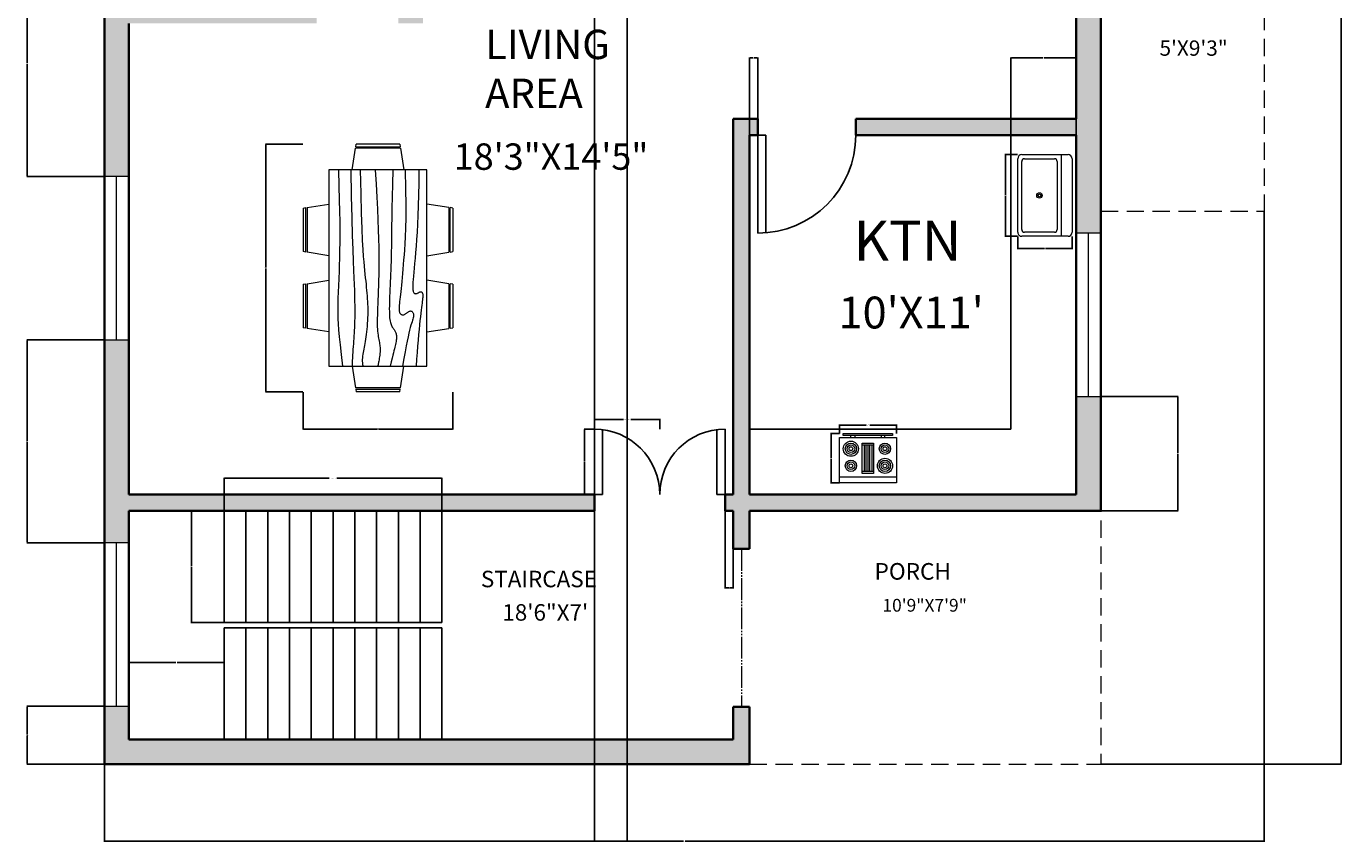
# Model space of a CAD drawing. Units: inches. Extents: x 60 to 543, y 115 to 735.
# Tile 1 of 2: x 60 to 543, y 115 to 415. Entities that reach past the tile are written whole.
import ezdxf

# ---------------------------------------------------------------- set-up
doc = ezdxf.new("R2010")
doc.units = ezdxf.units.IN
doc.linetypes.add('DASHED2', pattern=[9.525, 6.35, -3.175])
doc.linetypes.add('JIS_09_08', pattern=[10.75, 8, -0.55, 0.55, -0.55, 0.55, -0.55])
for name, color, linetype, lineweight in [('A-ANNO-DIMS', 2, 'Continuous', 18), ('A-AREA-IDEN', 7, 'Continuous', 18), ('A-DOOR', 4, 'Continuous', 25), ('A-EQPM', 9, 'Continuous', 18), ('A-FLOR-CASE', 8, 'Continuous', 25), ('A-FLOR-FIXT', 8, 'Continuous', 18), ('A-FLOR-OPEN', 8, 'JIS_09_08', 18), ('A-FLOR-OVHD', 8, 'DASHED2', 18), ('A-FLOR-STRS', 7, 'Continuous', 25), ('A-FURN', 8, 'Continuous', 18), ('A-GLAZ', 3, 'Continuous', 18), ('A-WALL', 7, 'Continuous', 35)]:
    doc.layers.add(name, color=color, linetype=linetype, lineweight=lineweight)
doc.layers.add('A-WALL-PATT', color=18, linetype='Continuous', lineweight=13, true_color=0x000000)
doc.styles.get("Standard").update_dxf_attribs({"font": 'arial.ttf'})
doc.dimstyles.get("Standard").update_dxf_attribs({"dimtxt": 0.18, "dimasz": 0.18, "dimexe": 0.18, "dimexo": 0.0625, "dimgap": 0.09, "dimtad": 0, "dimtih": 1, "dimtoh": 1, "dimdec": 4, "dimzin": 0, "dimdsep": 46, "dimtxsty": 'Standard', "dimcen": 0.09, "dimadec": 0, "dimazin": 0, "dimtfac": 1, "dimtdec": 4, "dimtofl": 0, "dimtmove": 0, "dimatfit": 3, "dimfxl": 1, "dimtolj": 1, "dimtzin": 0, "dimarcsym": 0})

# ---------------------------------------------------------------- blocks, each defined once
blk = doc.blocks.new('Dining Set - 36 x 72 in.')
for p, q in [((-22.2343, 26.00059), (-23.4847, 17.99762)), ((-22.2304, 26), (-5.7608, 26)), ((-22, 27.5), (-22.1562, 26.50042)), ((-5.8416, 26.5), (-22.1534, 26.5)), ((-22, 27.5), (-6, 27.5)), ((-5.8437, 26.49966), (-6, 27.5)), ((-4.5152, 17.99762), (-5.7655, 25.99926)), ((5.7657, 26.00059), (4.5153, 17.99762)), ((5.7696, 26), (22.2392, 26)), ((6, 27.5), (5.8438, 26.50042)), ((22.1584, 26.5), (5.8466, 26.5)), ((6, 27.5), (22, 27.5)), ((22.1563, 26.49966), (22, 27.5)), ((23.4848, 17.99762), (22.2345, 25.99926)), ((36, 18), (-36, 18)), ((-36, 18), (-36, -18)), ((36, -18), (36, 18)), ((-45.5, 8), (-44.5004, 8.15617)), ((-45.5, 8), (-45.5, -8)), ((-44.5, -8.15843), (-44.5, 8.15338)), ((-44.0006, 8.23428), (-35.9976, 9.48474)), ((-44, 8.23041), (-44, -8.23915)), ((44.0006, 8.23428), (35.9976, 9.48474)), ((44, 8.23041), (44, -8.23915)), ((44.5, -8.15843), (44.5, 8.15338)), ((45.5, 8), (44.5005, 8.15617)), ((45.5, 8), (45.5, -8)), ((-44.4997, -8.15631), (-45.5, -8)), ((-35.9976, -9.48476), (-43.9993, -8.2345)), ((35.9976, -9.48476), (43.9993, -8.2345)), ((44.4997, -8.15631), (45.5, -8)), ((-36, -18), (36, -18)), ((-22.2343, -26.0006), (-23.4847, -17.99762)), ((-4.5152, -17.99762), (-5.7655, -25.99928)), ((5.7657, -26.0006), (4.5153, -17.99762)), ((23.4848, -17.99762), (22.2345, -25.99928)), ((-22.2304, -26), (-5.7608, -26)), ((-22, -27.5), (-22.1562, -26.50044)), ((-5.8416, -26.5), (-22.1534, -26.5)), ((-22, -27.5), (-6, -27.5)), ((-5.8437, -26.49967), (-6, -27.5)), ((5.7696, -26), (22.2392, -26)), ((6, -27.5), (5.8438, -26.50044)), ((22.1584, -26.5), (5.8466, -26.5)), ((6, -27.5), (22, -27.5)), ((22.1563, -26.49967), (22, -27.5))]:
    blk.add_line(p, q)
for points in [[(-36, 15), (-31.1772, 14.97754), (-26.8079, 14.91406), (-22.8538, 14.81543), (-19.276, 14.6875), (-16.0362, 14.53613), (-13.0957, 14.36718), (-10.4159, 14.18652), (-7.9583, 14), (-5.6904, 13.81315), (-3.6035, 13.63021), (-1.6954, 13.45508), (0.0365, 13.29166), (1.5945, 13.14388), (2.9811, 13.01562), (4.1988, 12.9108), (5.25, 12.83333), (6.1393, 12.78613), (6.8802, 12.76823), (7.4883, 12.77767), (7.9792, 12.8125), (8.3685, 12.87077), (8.6719, 12.95052), (8.9049, 13.0498), (9.0833, 13.16666), (9.2205, 13.29899), (9.3216, 13.44401), (9.3895, 13.59879), (9.4271, 13.76041), (9.4373, 13.92594), (9.4232, 14.09245), (9.3875, 14.257), (9.3333, 14.41666), (9.2638, 14.56917), (9.1836, 14.71484), (9.0975, 14.85465), (9.0104, 14.98958), (8.9272, 15.1206), (8.8529, 15.2487), (8.7922, 15.37483), (8.75, 15.5), (8.7305, 15.62467), (8.7344, 15.74739), (8.7617, 15.86621), (8.8125, 15.97916), (8.8867, 16.08431), (8.9844, 16.17968), (9.1055, 16.26334), (9.25, 16.33333), (9.4189, 16.38802), (9.6172, 16.42708), (9.8506, 16.45052), (10.125, 16.45833), (10.4463, 16.45052), (10.8203, 16.42708), (11.2529, 16.38802), (11.75, 16.33333), (12.3184, 16.26318), (12.9694, 16.17838), (13.7151, 16.07991), (14.5677, 15.96875), (15.5395, 15.84586), (16.6426, 15.71224), (17.8893, 15.56884), (19.2917, 15.41666), (20.859, 15.25667), (22.5879, 15.08984), (24.4721, 14.91715), (26.5052, 14.73958), (28.6809, 14.5581), (30.9929, 14.3737), (33.4347, 14.18733), (36, 14)], [(-36, 10), (-28.9766, 10.14274), (-23.1725, 10.20442), (-18.4241, 10.19775), (-14.5677, 10.13541), (-11.4399, 10.03011), (-8.877, 9.89453), (-6.7154, 9.74137), (-4.7917, 9.58333), (-2.9698, 9.43082), (-1.2246, 9.28515), (0.4415, 9.14534), (2.026, 9.01041), (3.5266, 8.87939), (4.9408, 8.7513), (6.266, 8.62516), (7.5, 8.5), (8.6411, 8.37549), (9.6914, 8.2539), (10.6538, 8.13818), (11.5312, 8.03125), (12.3267, 7.93603), (13.043, 7.85547), (13.6831, 7.79248), (14.25, 7.75), (14.7471, 7.7303), (15.1797, 7.73307), (15.5537, 7.75732), (15.875, 7.80208), (16.1494, 7.86637), (16.3828, 7.94922), (16.5811, 8.04964), (16.75, 8.16666), (16.8944, 8.29915), (17.0143, 8.44531), (17.1089, 8.60319), (17.1771, 8.77083), (17.218, 8.94629), (17.2305, 9.1276), (17.2137, 9.31282), (17.1667, 9.5), (17.0895, 9.6875), (16.987, 9.875), (16.8649, 10.0625), (16.7292, 10.25), (16.5856, 10.4375), (16.4401, 10.625), (16.2985, 10.8125), (16.1667, 11), (16.05, 11.18733), (15.9518, 11.3737), (15.8752, 11.5581), (15.8229, 11.73958), (15.798, 11.91715), (15.8034, 12.08984), (15.842, 12.25667), (15.9167, 12.41666), (16.0295, 12.56836), (16.1784, 12.70833), (16.3605, 12.83268), (16.5729, 12.9375), (16.8127, 13.01888), (17.0768, 13.07291), (17.3625, 13.0957), (17.6667, 13.08333), (17.9894, 13.03312), (18.3418, 12.94726), (18.7382, 12.82918), (19.1927, 12.68229), (19.7195, 12.51001), (20.3327, 12.31575), (21.0465, 12.10294), (21.875, 11.875), (22.8357, 11.63354), (23.959, 11.37304), (25.2786, 11.08618), (26.8282, 10.76562), (28.6414, 10.40405), (30.752, 9.99414), (33.1936, 9.52856), (36, 9)], [(-36, 5.5), (-30.7157, 5.3348), (-26.069, 5.20963), (-21.9946, 5.11767), (-18.4271, 5.05208), (-15.3009, 5.00602), (-12.5508, 4.97265), (-10.1112, 4.94515), (-7.9167, 4.91666), (-5.909, 4.88167), (-4.0586, 4.83984), (-2.3429, 4.79215), (-0.7396, 4.73958), (0.7739, 4.6831), (2.22, 4.6237), (3.6213, 4.56233), (5, 4.5), (6.373, 4.43782), (7.7344, 4.3776), (9.0723, 4.32129), (10.375, 4.27083), (11.6309, 4.22819), (12.8281, 4.19531), (13.9551, 4.17415), (15, 4.16666), (15.954, 4.17448), (16.819, 4.19791), (17.6001, 4.23698), (18.3021, 4.29166), (18.9299, 4.36198), (19.4883, 4.44791), (19.9823, 4.54948), (20.4167, 4.66666), (20.7969, 4.79899), (21.1302, 4.94401), (21.4245, 5.09879), (21.6875, 5.26041), (21.9271, 5.42594), (22.1511, 5.59245), (22.3672, 5.757), (22.5834, 5.91666), (22.8065, 6.06868), (23.0404, 6.21093), (23.2879, 6.34147), (23.5521, 6.45833), (23.8358, 6.55957), (24.142, 6.64323), (24.4735, 6.70735), (24.8334, 6.75), (25.2235, 6.76969), (25.642, 6.76692), (26.0858, 6.74267), (26.5521, 6.69791), (27.0379, 6.63362), (27.5404, 6.55078), (28.0565, 6.45036), (28.5834, 6.33333), (29.1242, 6.19987), (29.7071, 6.04687), (30.3661, 5.87044), (31.1354, 5.66666), (32.0493, 5.43164), (33.142, 5.16146), (34.4475, 4.85221), (36, 4.5)], [(-36, -1), (-30.7915, -0.6591), (-26.0195, -0.38216), (-21.6519, -0.16284), (-17.6563, 0.00521), (-14.0005, 0.12833), (-10.6523, 0.21289), (-7.5796, 0.26522), (-4.75, 0.29166), (-2.134, 0.29793), (0.2878, 0.28711), (2.5317, 0.26163), (4.6146, 0.22396), (6.5529, 0.17651), (8.3633, 0.12174), (10.0623, 0.06209), (11.6667, 0), (13.1899, -0.06201), (14.6341, -0.1211), (15.9982, -0.17432), (17.2813, -0.21875), (18.4823, -0.25147), (19.6003, -0.26953), (20.6343, -0.27002), (21.5834, -0.25), (22.4481, -0.20768), (23.2357, -0.14584), (23.9549, -0.06836), (24.6146, 0.02083), (25.2235, 0.11784), (25.7904, 0.21875), (26.3241, 0.31966), (26.8334, 0.41666), (27.3265, 0.50618), (27.8099, 0.58593), (28.2894, 0.65397), (28.7709, 0.70833), (29.2601, 0.74707), (29.763, 0.76823), (30.2855, 0.76985), (30.8334, 0.75), (31.4088, 0.70784), (31.9994, 0.64713), (32.589, 0.57275), (33.1615, 0.48958), (33.7008, 0.4025), (34.1908, 0.3164), (34.6153, 0.23616), (34.9584, 0.16666), (35.2099, 0.11165), (35.3848, 0.07031), (35.504, 0.04069), (35.5886, 0.02083), (35.6594, 0.00879), (35.7377, 0.0026), (35.8442, 0.00032), (36, 0)], [(-36, -6.5), (-27.1843, -6.31267), (-20.084, -6.1263), (-14.469, -5.9419), (-10.1094, -5.76042), (-6.7752, -5.58285), (-4.2363, -5.41016), (-2.2629, -5.24333), (-0.625, -5.08334), (0.8708, -4.93099), (2.2715, -4.78646), (3.5872, -4.64974), (4.8281, -4.52084), (6.0046, -4.39974), (7.127, -4.28646), (8.2053, -4.18099), (9.25, -4.08334), (10.2705, -3.99382), (11.2734, -3.91407), (12.2647, -3.84603), (13.25, -3.79167), (14.2354, -3.75293), (15.2266, -3.73177), (16.2295, -3.73015), (17.25, -3.75), (18.2912, -3.79248), (19.3451, -3.85547), (20.4009, -3.93604), (21.4479, -4.03125), (22.4754, -4.13819), (23.4727, -4.25391), (24.4289, -4.37549), (25.3334, -4.5), (26.1785, -4.62492), (26.9694, -4.74935), (27.7145, -4.87281), (28.4219, -4.99479), (29.1, -5.11483), (29.7572, -5.23242), (30.4016, -5.34709), (31.0417, -5.45834), (31.6837, -5.56437), (32.3262, -5.65821), (32.9658, -5.73153), (33.599, -5.77604), (34.2224, -5.78345), (34.8327, -5.74545), (35.4264, -5.65373), (36, -5.5)], [(-36, -10), (-26.4022, -9.81299), (-18.4675, -9.62891), (-11.9839, -9.45069), (-6.7396, -9.28125), (-2.5226, -9.12354), (0.8789, -8.98047), (3.6769, -8.85498), (6.0833, -8.75), (8.2767, -8.66765), (10.3021, -8.60677), (12.1712, -8.56543), (13.8958, -8.54167), (15.4876, -8.53353), (16.9583, -8.53907), (18.3197, -8.55632), (19.5834, -8.58334), (20.7616, -8.61841), (21.8685, -8.66081), (22.9188, -8.71004), (23.9271, -8.76563), (24.9081, -8.82707), (25.8763, -8.89388), (26.8465, -8.96558), (27.8334, -9.04167), (28.8474, -9.12118), (29.8828, -9.20117), (30.93, -9.27824), (31.9792, -9.34896), (33.0205, -9.40991), (34.0443, -9.45768), (35.0407, -9.48885), (36, -9.5)], [(-36, -14.5), (-30.0881, -14.33513), (-25.0332, -14.21224), (-20.7312, -14.12647), (-17.0781, -14.07292), (-13.97, -14.04671), (-11.3027, -14.04297), (-8.9724, -14.05681), (-6.875, -14.08334), (-4.9224, -14.11833), (-3.0905, -14.16016), (-1.3709, -14.20785), (0.2448, -14.26042), (1.7647, -14.3169), (3.1973, -14.3763), (4.5507, -14.43767), (5.8333, -14.5), (7.0554, -14.5621), (8.235, -14.62175), (9.3922, -14.67652), (10.5469, -14.72396), (11.7192, -14.76164), (12.929, -14.78711), (14.1965, -14.79794), (15.5417, -14.79167), (16.9933, -14.76424), (18.6152, -14.70508), (20.4804, -14.60197), (22.6615, -14.44271), (25.2312, -14.21509), (28.2624, -13.9069), (31.8277, -13.50594), (36, -13)]]:
    blk.add_lwpolyline(points)
blk = doc.blocks.new('Sink-single - 30 in top')
blk.add_line((-15, -3.999996), (15, -3.999996))
for points in [[(-13.5, 0), (13.5, 0)], [(-15, -18.499996), (-15, -1.5)], [(15, -1.5), (15, -18.499996)], [(-13.5, -17.499996), (-13.5, -6.499996)], [(-12.5, -5.499996), (12.5, -5.499996)], [(13.5, -6.499996), (13.5, -17.499996)], [(12.5, -18.499996), (-12.5, -18.499996)], [(13.5, -19.999996), (-13.5, -19.999996)]]:
    blk.add_lwpolyline(points)
for radius in [1, 0.5]:
    blk.add_circle((0, -11.999996), radius)
for centre, radius, start, end in [((-13.5, -1.5), 1.5, 90, 180), ((13.5, -1.5), 1.5, 0, 90), ((-12.5, -6.499996), 1, 90, 180), ((12.5, -6.499996), 1, 0, 90), ((-13.5, -18.499996), 1.5, 180, 270), ((-12.5, -17.499996), 1, 180, 270), ((12.5, -17.499996), 1, 270, 0), ((13.5, -18.499996), 1.5, 270, 0)]:
    blk.add_arc(centre, radius, start, end)
blk = doc.blocks.new('Range-Oven - 30 in top')
for p, q in [((0, -3), (30, -3)), ((12, -6), (18, -6)), ((13, -20), (13, -6)), ((14, -6), (14, -20)), ((15, -20), (15, -6)), ((16, -6), (16, -20)), ((17, -20), (17, -6)), ((18, -20), (12, -20)), ((6, -24), (6, -25)), ((8, -25), (8, -24)), ((22, -25), (22, -24)), ((24, -24), (24, -25))]:
    blk.add_line(p, q)
for points in [[(0, -24), (0, 0), (30, 0), (30, -24)], [(12, -21), (12, -5), (18, -5), (18, -21)], [(2, -26), (2, -25), (28, -25), (28, -26)]]:
    blk.add_lwpolyline(points, close=True)
for centre, radius in [((6, -9), 4), ((6, -9), 3), ((24, -9), 3), ((6, -9), 2), ((6, -9), 1), ((24, -9), 2), ((24, -9), 1), ((6, -18), 3), ((6, -18), 2), ((6, -18), 1), ((24, -18), 4), ((24, -18), 3), ((24, -18), 2), ((24, -18), 1)]:
    blk.add_circle(centre, radius)
blk = doc.blocks.new('DOOR-SWING-36IN')
for p, q in [((0, 0), (0, 36)), ((0, 36), (3, 36)), ((3, 0), (3, 36))]:
    blk.add_line(p, q)
blk.add_arc((0, 36), 36, 270, 0)
blk = doc.blocks.new('DOOR-ENTRY-LEAF-24IN')
for p, q in [((0, 24), (0, 0)), ((3, 24), (3, 0)), ((0, 0), (3, 0))]:
    blk.add_line(p, q)
blk.add_arc((0, 0), 24, 0, 90)
blk = doc.blocks.new('WINDOW-60IN')
for p, q in [((9, 60), (0, 60)), ((0, 60), (0, 0)), ((4.5, 0), (4.5, 60)), ((9, 0), (9, 60)), ((0, 0), (9, 0))]:
    blk.add_line(p, q)
blk = doc.blocks.new('STAIR-FLIGHT-80X41IN')
for p, q in [((0, 41), (0, 0)), ((8, 41), (8, 0)), ((16, 41), (16, 0)), ((24, 41), (24, 0)), ((32, 41), (32, 0)), ((40, 41), (40, 0)), ((48, 41), (48, 0)), ((56, 41), (56, 0)), ((64, 41), (64, 0)), ((72, 41), (72, 0)), ((80, 41), (80, 0)), ((0, 0), (80, 0))]:
    blk.add_line(p, q)
blk = doc.blocks.new('*D27')
at = {"layer": 'A-ANNO-DIMS', "color": 0, "lineweight": -2, "transparency": 16777216}
for p, q in [((268.39, 267.03), (268.39, 270.75)), ((292.39, 267.03), (292.39, 270.75)), ((268.57, 270.57), (279.06, 270.57)), ((292.21, 270.57), (281.73, 270.57))]:
    blk.add_line(p, q, dxfattribs=at)
at = {"layer": 'A-ANNO-DIMS', "color": 0, "transparency": 16777216}
for points in [[(268.57, 270.6), (268.57, 270.54), (268.39, 270.57)], [(292.21, 270.6), (292.21, 270.54), (292.39, 270.57)]]:
    blk.add_solid(points, dxfattribs=at)
at = {"layer": 'Defpoints', "color": 0, "transparency": 16777216}
for p in [(268.39, 266.97), (292.39, 270.57), (292.39, 266.97)]:
    blk.add_point(p, dxfattribs=at)
at = {"layer": 'A-ANNO-DIMS', "color": 0, "transparency": 16777216, "insert": (280.39, 270.57), "char_height": 0.18, "attachment_point": 5}
blk.add_mtext('\\A1;ENTRY LEAF 24 TYP.', dxfattribs=at)
blk = doc.blocks.new('*D28')
at = {"layer": 'A-ANNO-DIMS', "color": 0, "lineweight": -2, "transparency": 16777216}
for p, q in [((268.33, 266.97), (264.61, 266.97)), ((264.79, 266.79), (264.79, 255.15)), ((264.79, 243.15), (264.79, 254.79)), ((268.33, 242.97), (264.61, 242.97))]:
    blk.add_line(p, q, dxfattribs=at)
at = {"layer": 'A-ANNO-DIMS', "color": 0, "transparency": 16777216}
for points in [[(264.76, 266.79), (264.82, 266.79), (264.79, 266.97)], [(264.76, 243.15), (264.82, 243.15), (264.79, 242.97)]]:
    blk.add_solid(points, dxfattribs=at)
at = {"layer": 'Defpoints', "color": 0, "transparency": 16777216}
for p in [(264.79, 266.97), (268.39, 266.97), (268.39, 242.97)]:
    blk.add_point(p, dxfattribs=at)
at = {"layer": 'A-ANNO-DIMS', "color": 0, "transparency": 16777216, "insert": (264.79, 254.97), "char_height": 0.18, "attachment_point": 5}
blk.add_mtext('\\A1;24 TYP.', dxfattribs=at)
blk = doc.blocks.new('*D29')
at = {"layer": 'A-ANNO-DIMS', "color": 0, "lineweight": -2, "transparency": 16777216}
for p, q in [((132.39, 237.03), (132.39, 249.15)), ((132.57, 248.97), (170.98, 248.97)), ((212.21, 248.97), (173.81, 248.97)), ((212.39, 237.03), (212.39, 249.15))]:
    blk.add_line(p, q, dxfattribs=at)
at = {"layer": 'A-ANNO-DIMS', "color": 0, "transparency": 16777216}
for points in [[(132.57, 249), (132.57, 248.94), (132.39, 248.97)], [(212.21, 249), (212.21, 248.94), (212.39, 248.97)]]:
    blk.add_solid(points, dxfattribs=at)
at = {"layer": 'Defpoints', "color": 0, "transparency": 16777216}
for p in [(212.39, 248.97), (132.39, 236.97), (212.39, 236.97)]:
    blk.add_point(p, dxfattribs=at)
at = {"layer": 'A-ANNO-DIMS', "color": 0, "transparency": 16777216, "insert": (172.39, 248.97), "char_height": 0.18, "attachment_point": 5}
blk.add_mtext('\\A1;STAIR FLIGHT 80 TYP.', dxfattribs=at)
blk = doc.blocks.new('*D30')
at = {"layer": 'A-ANNO-DIMS', "color": 0, "lineweight": -2, "transparency": 16777216}
for p, q in [((132.33, 236.97), (120.21, 236.97)), ((120.39, 236.79), (120.39, 216.65)), ((120.39, 196.15), (120.39, 216.29)), ((132.33, 195.97), (120.21, 195.97))]:
    blk.add_line(p, q, dxfattribs=at)
at = {"layer": 'A-ANNO-DIMS', "color": 0, "transparency": 16777216}
for points in [[(120.36, 236.79), (120.42, 236.79), (120.39, 236.97)], [(120.36, 196.15), (120.42, 196.15), (120.39, 195.97)]]:
    blk.add_solid(points, dxfattribs=at)
at = {"layer": 'Defpoints', "color": 0, "transparency": 16777216}
for p in [(120.39, 236.97), (132.39, 236.97), (132.39, 195.97)]:
    blk.add_point(p, dxfattribs=at)
at = {"layer": 'A-ANNO-DIMS', "color": 0, "transparency": 16777216, "insert": (120.39, 216.47), "char_height": 0.18, "attachment_point": 5}
blk.add_mtext('\\A1;41 TYP.', dxfattribs=at)
blk = doc.blocks.new('*D31')
at = {"layer": 'A-ANNO-DIMS', "color": 0, "lineweight": -2, "transparency": 16777216}
for p, q in [((161.34, 371.66), (147.57, 371.66)), ((147.75, 371.48), (147.75, 326.34)), ((147.75, 280.84), (147.75, 325.98)), ((161.34, 280.66), (147.57, 280.66))]:
    blk.add_line(p, q, dxfattribs=at)
at = {"layer": 'A-ANNO-DIMS', "color": 0, "transparency": 16777216}
for points in [[(147.72, 371.48), (147.78, 371.48), (147.75, 371.66)], [(147.72, 280.84), (147.78, 280.84), (147.75, 280.66)]]:
    blk.add_solid(points, dxfattribs=at)
at = {"layer": 'Defpoints', "color": 0, "transparency": 16777216}
for p in [(161.4, 371.66), (147.75, 280.66), (161.4, 280.66)]:
    blk.add_point(p, dxfattribs=at)
at = {"layer": 'A-ANNO-DIMS', "color": 0, "transparency": 16777216, "insert": (147.75, 326.16), "char_height": 0.18, "attachment_point": 5}
blk.add_mtext('\\A1;DINING SET 91', dxfattribs=at)
blk = doc.blocks.new('*D32')
at = {"layer": 'A-ANNO-DIMS', "color": 0, "lineweight": -2, "transparency": 16777216}
for p, q in [((161.4, 280.6), (161.4, 266.83)), ((216.4, 280.6), (216.4, 266.83)), ((161.58, 267.01), (188.68, 267.01)), ((216.22, 267.01), (189.12, 267.01))]:
    blk.add_line(p, q, dxfattribs=at)
at = {"layer": 'A-ANNO-DIMS', "color": 0, "transparency": 16777216}
for points in [[(161.58, 267.04), (161.58, 266.98), (161.4, 267.01)], [(216.22, 267.04), (216.22, 266.98), (216.4, 267.01)]]:
    blk.add_solid(points, dxfattribs=at)
at = {"layer": 'Defpoints', "color": 0, "transparency": 16777216}
for p in [(161.4, 280.66), (216.4, 280.66), (216.4, 267.01)]:
    blk.add_point(p, dxfattribs=at)
at = {"layer": 'A-ANNO-DIMS', "color": 0, "transparency": 16777216, "insert": (188.9, 267.01), "char_height": 0.18, "attachment_point": 5}
blk.add_mtext('\\A1;55', dxfattribs=at)
blk = doc.blocks.new('*D33')
at = {"layer": 'A-ANNO-DIMS', "color": 0, "lineweight": -2, "transparency": 16777216}
for p, q in [((423.82, 367.78), (419.21, 367.78)), ((419.39, 367.6), (419.39, 352.96)), ((419.39, 337.96), (419.39, 352.6)), ((423.82, 337.78), (419.21, 337.78))]:
    blk.add_line(p, q, dxfattribs=at)
at = {"layer": 'A-ANNO-DIMS', "color": 0, "transparency": 16777216}
for points in [[(419.36, 367.6), (419.42, 367.6), (419.39, 367.78)], [(419.36, 337.96), (419.42, 337.96), (419.39, 337.78)]]:
    blk.add_solid(points, dxfattribs=at)
at = {"layer": 'Defpoints', "color": 0, "transparency": 16777216}
for p in [(423.89, 367.78), (419.39, 337.78), (423.89, 337.78)]:
    blk.add_point(p, dxfattribs=at)
at = {"layer": 'A-ANNO-DIMS', "color": 0, "transparency": 16777216, "insert": (419.39, 352.78), "char_height": 0.18, "attachment_point": 5}
blk.add_mtext('\\A1;SINK 30', dxfattribs=at)
blk = doc.blocks.new('*D34')
at = {"layer": 'A-ANNO-DIMS', "color": 0, "lineweight": -2, "transparency": 16777216}
for p, q in [((423.89, 337.72), (423.89, 333.1)), ((443.89, 337.72), (443.89, 333.1)), ((424.07, 333.28), (433.67, 333.28)), ((443.71, 333.28), (434.11, 333.28))]:
    blk.add_line(p, q, dxfattribs=at)
at = {"layer": 'A-ANNO-DIMS', "color": 0, "transparency": 16777216}
for points in [[(424.07, 333.31), (424.07, 333.25), (423.89, 333.28)], [(443.71, 333.31), (443.71, 333.25), (443.89, 333.28)]]:
    blk.add_solid(points, dxfattribs=at)
at = {"layer": 'Defpoints', "color": 0, "transparency": 16777216}
for p in [(423.89, 337.78), (443.89, 337.78), (443.89, 333.28)]:
    blk.add_point(p, dxfattribs=at)
at = {"layer": 'A-ANNO-DIMS', "color": 0, "transparency": 16777216, "insert": (433.89, 333.28), "char_height": 0.18, "attachment_point": 5}
blk.add_mtext('\\A1;20', dxfattribs=at)
blk = doc.blocks.new('*D35')
at = {"layer": 'A-ANNO-DIMS', "color": 0, "lineweight": -2, "transparency": 16777216}
for p, q in [((358.44, 265.41), (358.44, 268.66)), ((358.62, 268.48), (368.2, 268.48)), ((379.13, 268.48), (369.55, 268.48)), ((379.31, 265.41), (379.31, 268.66))]:
    blk.add_line(p, q, dxfattribs=at)
at = {"layer": 'A-ANNO-DIMS', "color": 0, "transparency": 16777216}
for points in [[(358.62, 268.51), (358.62, 268.45), (358.44, 268.48)], [(379.13, 268.51), (379.13, 268.45), (379.31, 268.48)]]:
    blk.add_solid(points, dxfattribs=at)
at = {"layer": 'Defpoints', "color": 0, "transparency": 16777216}
for p in [(358.44, 268.48), (358.44, 265.35), (379.31, 265.35)]:
    blk.add_point(p, dxfattribs=at)
at = {"layer": 'A-ANNO-DIMS', "color": 0, "transparency": 16777216, "insert": (368.88, 268.48), "char_height": 0.18, "attachment_point": 5}
blk.add_mtext('\\A1;RANGE 21', dxfattribs=at)
blk = doc.blocks.new('*D36')
at = {"layer": 'A-ANNO-DIMS', "color": 0, "lineweight": -2, "transparency": 16777216}
for p, q in [((358.38, 265.35), (355.13, 265.35)), ((355.31, 265.17), (355.31, 256.49)), ((355.31, 247.45), (355.31, 256.13)), ((358.38, 247.27), (355.13, 247.27))]:
    blk.add_line(p, q, dxfattribs=at)
at = {"layer": 'A-ANNO-DIMS', "color": 0, "transparency": 16777216}
for points in [[(355.28, 265.17), (355.34, 265.17), (355.31, 265.35)], [(355.28, 247.45), (355.34, 247.45), (355.31, 247.27)]]:
    blk.add_solid(points, dxfattribs=at)
at = {"layer": 'Defpoints', "color": 0, "transparency": 16777216}
for p in [(358.44, 265.35), (355.31, 247.27), (358.44, 247.27)]:
    blk.add_point(p, dxfattribs=at)
at = {"layer": 'A-ANNO-DIMS', "color": 0, "transparency": 16777216, "insert": (355.31, 256.31), "char_height": 0.18, "attachment_point": 5}
blk.add_mtext('\\A1;18', dxfattribs=at)
blk = doc.blocks.new('*D37')
at = {"layer": 'A-ANNO-DIMS', "color": 0, "lineweight": -2, "transparency": 16777216}
for p, q in [((514.39, 346.91), (514.39, 115.49)), ((88.39, 143.91), (88.39, 115.49)), ((88.57, 115.67), (301.1, 115.67)), ((514.21, 115.67), (301.69, 115.67))]:
    blk.add_line(p, q, dxfattribs=at)
at = {"layer": 'A-ANNO-DIMS', "color": 0, "transparency": 16777216}
for points in [[(88.57, 115.7), (88.57, 115.64), (88.39, 115.67)], [(514.21, 115.7), (514.21, 115.64), (514.39, 115.67)]]:
    blk.add_solid(points, dxfattribs=at)
at = {"layer": 'Defpoints', "color": 0, "transparency": 16777216}
for p in [(514.39, 346.97), (88.39, 143.97), (514.39, 115.67)]:
    blk.add_point(p, dxfattribs=at)
at = {"layer": 'A-ANNO-DIMS', "color": 0, "transparency": 16777216, "insert": (301.39, 115.67), "char_height": 0.18, "attachment_point": 5}
blk.add_mtext('\\A1;426', dxfattribs=at)
blk = doc.blocks.new('*D38')
at = {"layer": 'A-ANNO-DIMS', "color": 0, "lineweight": -2, "transparency": 16777216}
for p, q in [((454.46, 706.97), (542.87, 706.97)), ((542.69, 706.79), (542.69, 425.65)), ((542.69, 144.15), (542.69, 425.29)), ((454.46, 143.97), (542.87, 143.97))]:
    blk.add_line(p, q, dxfattribs=at)
at = {"layer": 'A-ANNO-DIMS', "color": 0, "transparency": 16777216}
for points in [[(542.66, 706.79), (542.72, 706.79), (542.69, 706.97)], [(542.66, 144.15), (542.72, 144.15), (542.69, 143.97)]]:
    blk.add_solid(points, dxfattribs=at)
at = {"layer": 'Defpoints', "color": 0, "transparency": 16777216}
for p in [(454.39, 706.97), (542.69, 706.97), (454.39, 143.97)]:
    blk.add_point(p, dxfattribs=at)
at = {"layer": 'A-ANNO-DIMS', "color": 0, "transparency": 16777216, "insert": (542.69, 425.47), "char_height": 0.18, "attachment_point": 5}
blk.add_mtext('\\A1;563', dxfattribs=at)
blk = doc.blocks.new('*D40')
at = {"layer": 'A-ANNO-DIMS', "color": 0, "lineweight": -2, "transparency": 16777216}
for p, q in [((88.33, 165.24), (59.91, 165.24)), ((60.09, 165.06), (60.09, 154.79)), ((60.09, 144.15), (60.09, 154.42)), ((88.33, 143.97), (59.91, 143.97))]:
    blk.add_line(p, q, dxfattribs=at)
at = {"layer": 'A-ANNO-DIMS', "color": 0, "transparency": 16777216}
for points in [[(60.06, 165.06), (60.12, 165.06), (60.09, 165.24)], [(60.06, 144.15), (60.12, 144.15), (60.09, 143.97)]]:
    blk.add_solid(points, dxfattribs=at)
at = {"layer": 'Defpoints', "color": 0, "transparency": 16777216}
for p in [(60.09, 165.24), (88.39, 165.24), (88.39, 143.97)]:
    blk.add_point(p, dxfattribs=at)
at = {"layer": 'A-ANNO-DIMS', "color": 0, "transparency": 16777216, "insert": (60.09, 154.6), "char_height": 0.18, "attachment_point": 5}
blk.add_mtext('\\A1;21.268', dxfattribs=at)
blk = doc.blocks.new('*D41')
at = {"layer": 'A-ANNO-DIMS', "color": 0, "lineweight": -2, "transparency": 16777216}
for p, q in [((88.33, 299.74), (59.91, 299.74)), ((60.09, 299.56), (60.09, 262.67)), ((60.09, 225.42), (60.09, 262.31)), ((88.33, 225.24), (59.91, 225.24))]:
    blk.add_line(p, q, dxfattribs=at)
at = {"layer": 'A-ANNO-DIMS', "color": 0, "transparency": 16777216}
for points in [[(60.06, 299.56), (60.12, 299.56), (60.09, 299.74)], [(60.06, 225.42), (60.12, 225.42), (60.09, 225.24)]]:
    blk.add_solid(points, dxfattribs=at)
at = {"layer": 'Defpoints', "color": 0, "transparency": 16777216}
for p in [(60.09, 299.74), (88.39, 299.74), (88.39, 225.24)]:
    blk.add_point(p, dxfattribs=at)
at = {"layer": 'A-ANNO-DIMS', "color": 0, "transparency": 16777216, "insert": (60.09, 262.49), "char_height": 0.18, "attachment_point": 5}
blk.add_mtext('\\A1;74.5', dxfattribs=at)
blk = doc.blocks.new('*D42')
at = {"layer": 'A-ANNO-DIMS', "color": 0, "lineweight": -2, "transparency": 16777216}
for p, q in [((88.33, 442.97), (59.91, 442.97)), ((60.09, 442.79), (60.09, 401.54)), ((60.09, 359.92), (60.09, 401.17)), ((88.33, 359.74), (59.91, 359.74))]:
    blk.add_line(p, q, dxfattribs=at)
at = {"layer": 'A-ANNO-DIMS', "color": 0, "transparency": 16777216}
for points in [[(60.06, 442.79), (60.12, 442.79), (60.09, 442.97)], [(60.06, 359.92), (60.12, 359.92), (60.09, 359.74)]]:
    blk.add_solid(points, dxfattribs=at)
at = {"layer": 'Defpoints', "color": 0, "transparency": 16777216}
for p in [(60.09, 442.97), (88.39, 442.97), (88.39, 359.74)]:
    blk.add_point(p, dxfattribs=at)
at = {"layer": 'A-ANNO-DIMS', "color": 0, "transparency": 16777216, "insert": (60.09, 401.35), "char_height": 0.18, "attachment_point": 5}
blk.add_mtext('\\A1;83.23', dxfattribs=at)
blk = doc.blocks.new('*D46')
at = {"layer": 'A-ANNO-DIMS', "color": 0, "lineweight": -2, "transparency": 16777216}
for p, q in [((454.46, 278.97), (482.87, 278.97)), ((482.69, 278.79), (482.69, 258.15)), ((482.69, 237.15), (482.69, 257.79)), ((454.46, 236.97), (482.87, 236.97))]:
    blk.add_line(p, q, dxfattribs=at)
at = {"layer": 'A-ANNO-DIMS', "color": 0, "transparency": 16777216}
for points in [[(482.66, 278.79), (482.72, 278.79), (482.69, 278.97)], [(482.66, 237.15), (482.72, 237.15), (482.69, 236.97)]]:
    blk.add_solid(points, dxfattribs=at)
at = {"layer": 'Defpoints', "color": 0, "transparency": 16777216}
for p in [(454.39, 278.97), (454.39, 236.97), (482.69, 236.97)]:
    blk.add_point(p, dxfattribs=at)
at = {"layer": 'A-ANNO-DIMS', "color": 0, "transparency": 16777216, "insert": (482.69, 257.97), "char_height": 0.18, "attachment_point": 5}
blk.add_mtext('\\A1;42', dxfattribs=at)
blk = doc.blocks.new('*D50')
at = {"layer": 'A-ANNO-DIMS', "color": 0, "lineweight": -2, "transparency": 16777216}
for p, q in [((316.39, 236.91), (316.39, 208.49)), ((319.39, 236.91), (319.39, 208.49)), ((316.57, 208.67), (317.74, 208.67)), ((319.21, 208.67), (318.04, 208.67))]:
    blk.add_line(p, q, dxfattribs=at)
at = {"layer": 'A-ANNO-DIMS', "color": 0, "transparency": 16777216}
for points in [[(316.57, 208.7), (316.57, 208.64), (316.39, 208.67)], [(319.21, 208.7), (319.21, 208.64), (319.39, 208.67)]]:
    blk.add_solid(points, dxfattribs=at)
at = {"layer": 'Defpoints', "color": 0, "transparency": 16777216}
for p in [(316.39, 236.97), (319.39, 236.97), (316.39, 208.67)]:
    blk.add_point(p, dxfattribs=at)
at = {"layer": 'A-ANNO-DIMS', "color": 0, "transparency": 16777216, "insert": (317.89, 208.67), "char_height": 0.18, "attachment_point": 5}
blk.add_mtext('\\A1;3', dxfattribs=at)
blk = doc.blocks.new('*D52')
at = {"layer": 'A-ANNO-DIMS', "color": 0, "lineweight": -2, "transparency": 16777216}
for p, q in [((325.39, 375.03), (325.39, 403.45)), ((325.57, 403.27), (326.74, 403.27)), ((328.21, 403.27), (327.04, 403.27)), ((328.39, 375.03), (328.39, 403.45))]:
    blk.add_line(p, q, dxfattribs=at)
at = {"layer": 'A-ANNO-DIMS', "color": 0, "transparency": 16777216}
for points in [[(325.57, 403.3), (325.57, 403.24), (325.39, 403.27)], [(328.21, 403.3), (328.21, 403.24), (328.39, 403.27)]]:
    blk.add_solid(points, dxfattribs=at)
at = {"layer": 'Defpoints', "color": 0, "transparency": 16777216}
for p in [(328.39, 403.27), (325.39, 374.97), (328.39, 374.97)]:
    blk.add_point(p, dxfattribs=at)
at = {"layer": 'A-ANNO-DIMS', "color": 0, "transparency": 16777216, "insert": (326.89, 403.27), "char_height": 0.18, "attachment_point": 5}
blk.add_mtext('\\A1;3', dxfattribs=at)
blk = doc.blocks.new('*D53')
at = {"layer": 'A-ANNO-DIMS', "color": 0, "lineweight": -2, "transparency": 16777216}
for p, q in [((421.39, 375.03), (421.39, 403.45)), ((421.57, 403.27), (433.17, 403.27)), ((445.21, 403.27), (433.61, 403.27)), ((445.39, 375.03), (445.39, 403.45))]:
    blk.add_line(p, q, dxfattribs=at)
at = {"layer": 'A-ANNO-DIMS', "color": 0, "transparency": 16777216}
for points in [[(421.57, 403.3), (421.57, 403.24), (421.39, 403.27)], [(445.21, 403.3), (445.21, 403.24), (445.39, 403.27)]]:
    blk.add_solid(points, dxfattribs=at)
at = {"layer": 'Defpoints', "color": 0, "transparency": 16777216}
for p in [(445.39, 403.27), (421.39, 374.97), (445.39, 374.97)]:
    blk.add_point(p, dxfattribs=at)
at = {"layer": 'A-ANNO-DIMS', "color": 0, "transparency": 16777216, "insert": (433.39, 403.27), "char_height": 0.18, "attachment_point": 5}
blk.add_mtext('\\A1;24', dxfattribs=at)
blk = doc.blocks.new('*D54')
at = {"layer": 'A-ANNO-DIMS', "color": 0, "lineweight": -2, "transparency": 16777216}
for p, q in [((97.39, 153.03), (97.39, 181.45)), ((97.57, 181.27), (114.67, 181.27)), ((132.21, 181.27), (115.11, 181.27)), ((132.39, 153.03), (132.39, 181.45))]:
    blk.add_line(p, q, dxfattribs=at)
at = {"layer": 'A-ANNO-DIMS', "color": 0, "transparency": 16777216}
for points in [[(97.57, 181.3), (97.57, 181.24), (97.39, 181.27)], [(132.21, 181.3), (132.21, 181.24), (132.39, 181.27)]]:
    blk.add_solid(points, dxfattribs=at)
at = {"layer": 'Defpoints', "color": 0, "transparency": 16777216}
for p in [(132.39, 181.27), (97.39, 152.97), (132.39, 152.97)]:
    blk.add_point(p, dxfattribs=at)
at = {"layer": 'A-ANNO-DIMS', "color": 0, "transparency": 16777216, "insert": (114.89, 181.27), "char_height": 0.18, "attachment_point": 5}
blk.add_mtext('\\A1;35', dxfattribs=at)
blk = doc.blocks.new('*D55')
at = {"layer": 'A-ANNO-DIMS', "color": 0, "lineweight": -2, "transparency": 16777216}
for p, q in [((268.39, 559.91), (268.39, 115.49)), ((280.39, 559.91), (280.39, 115.49)), ((268.57, 115.67), (274.18, 115.67)), ((280.21, 115.67), (274.6, 115.67))]:
    blk.add_line(p, q, dxfattribs=at)
at = {"layer": 'A-ANNO-DIMS', "color": 0, "transparency": 16777216}
for points in [[(268.57, 115.7), (268.57, 115.64), (268.39, 115.67)], [(280.21, 115.7), (280.21, 115.64), (280.39, 115.67)]]:
    blk.add_solid(points, dxfattribs=at)
at = {"layer": 'Defpoints', "color": 0, "transparency": 16777216}
for p in [(268.39, 559.97), (280.39, 559.97), (280.39, 115.67)]:
    blk.add_point(p, dxfattribs=at)
at = {"layer": 'A-ANNO-DIMS', "color": 0, "transparency": 16777216, "insert": (274.39, 115.67), "char_height": 0.18, "attachment_point": 5}
blk.add_mtext('\\A1;12', dxfattribs=at)

msp = doc.modelspace()

# ---------------------------------------------------------------- hatches: boundary and pattern name
at = {"layer": 'A-WALL-PATT'}
h = msp.add_hatch(color=256, dxfattribs=at)
h.dxf.hatch_style = 1
h.paths.add_polyline_path([(454.3937, 706.9693), (277.3937, 706.9693), (271.3937, 706.9693), (88.3937, 706.9693), (88.3937, 681.945), (97.3937, 681.945), (97.3937, 697.9693), (271.3937, 697.9693), (271.3937, 565.9693), (268.3937, 565.9693), (268.3937, 559.9693), (271.3937, 559.9693), (277.3937, 559.9693), (280.3937, 559.9693), (280.3937, 565.9693), (277.3937, 565.9693), (277.3937, 697.9693), (445.3937, 697.9693), (445.3937, 681.945), (454.3937, 681.945)])
h.paths.add_polyline_path([(97.3937, 621.945), (88.3937, 621.945), (88.3937, 565.9693), (88.3937, 538.9693), (97.3937, 538.9693), (97.3937, 559.9693), (166.3937, 559.9693), (166.3937, 565.9693), (97.3937, 565.9693)])
h.paths.add_polyline_path([(454.3937, 621.945), (445.3937, 621.945), (445.3937, 565.9693), (382.3937, 565.9693), (382.3937, 559.9693), (445.3937, 559.9693), (445.3937, 523.9693), (454.3937, 523.9693), (454.3937, 559.9693), (454.3937, 565.9693)])
h.paths.add_polyline_path([(352.3937, 565.9693), (316.3937, 565.9693), (316.3937, 559.9693), (343.3937, 559.9693), (343.3937, 457.9693), (445.3937, 457.9693), (445.3937, 454.9693), (454.3937, 454.9693), (454.3937, 499.9693), (445.3937, 499.9693), (445.3937, 463.9693), (349.3937, 463.9693), (349.3937, 559.9693), (352.3937, 559.9693)])
h.paths.add_polyline_path([(232.3937, 565.9693), (196.3937, 565.9693), (196.3937, 559.9693), (199.3937, 559.9693), (199.3937, 493.9693), (97.3937, 493.9693), (97.3937, 514.9693), (88.3937, 514.9693), (88.3937, 466.9693), (97.3937, 466.9693), (97.3937, 487.9693), (199.3937, 487.9693), (199.3937, 421.9693), (196.3937, 421.9693), (196.3937, 415.9693), (199.3937, 415.9693), (205.3937, 415.9693), (205.3937, 421.9693), (205.3937, 493.9693), (205.3937, 559.9693), (232.3937, 559.9693)])
h.paths.add_polyline_path([(97.3937, 415.9693), (166.3937, 415.9693), (166.3937, 421.9693), (97.3937, 421.9693), (97.3937, 442.9693), (88.3937, 442.9693), (88.3937, 421.9693), (88.3937, 359.7372), (97.3937, 359.7372)])
h.paths.add_polyline_path([(97.3937, 299.7372), (88.3937, 299.7372), (88.3937, 225.2372), (97.3937, 225.2372), (97.3937, 236.9693), (199.3937, 236.9693), (268.3937, 236.9693), (268.3937, 242.9693), (199.3937, 242.9693), (97.3937, 242.9693)])
h.paths.add_polyline_path([(97.3937, 165.2372), (88.3937, 165.2372), (88.3937, 143.9693), (97.3937, 143.9693), (199.3937, 143.9693), (325.3937, 143.9693), (325.3937, 164.9693), (319.3937, 164.9693), (319.3937, 152.9693), (199.3937, 152.9693), (97.3937, 152.9693)])
h.paths.add_polyline_path([(454.3937, 242.9693), (454.3937, 278.9693), (445.3937, 278.9693), (445.3937, 242.9693), (325.3937, 242.9693), (325.3937, 374.9693), (328.3937, 374.9693), (328.3937, 380.9693), (319.3937, 380.9693), (319.3937, 242.9693), (316.3937, 242.9693), (316.3937, 236.9693), (319.3937, 236.9693), (319.3937, 222.9693), (325.3937, 222.9693), (325.3937, 236.9693), (454.3937, 236.9693)])
h.paths.add_polyline_path([(454.3937, 424.9693), (445.3937, 424.9693), (445.3937, 380.9693), (364.3937, 380.9693), (364.3937, 374.9693), (445.3937, 374.9693), (445.3937, 338.9693), (454.3937, 338.9693), (454.3937, 346.9693)])

# ---------------------------------------------------------------- linework, layer by layer
at = {"layer": 'A-FLOR-CASE'}
for p in [(421.3937, 374.9693), (325.3937, 266.9693)]:
    msp.add_line(p, (421.3937, 266.9693), dxfattribs=at)
at = {"layer": 'A-FLOR-OPEN'}
msp.add_line((322.3937, 222.9693), (322.3937, 164.9693), dxfattribs=at)
at = {"layer": 'A-FLOR-OVHD'}
for p, q in [((514.3937, 457.9693), (514.3937, 346.9693)), ((454.3937, 424.9693), (454.3937, 346.9693)), ((454.3937, 346.9693), (514.3937, 346.9693)), ((454.3937, 242.9693), (454.3937, 143.9693)), ((325.3937, 143.9693), (454.3937, 143.9693))]:
    msp.add_line(p, q, dxfattribs=at)
at = {"layer": 'A-WALL'}
for p, q in [((88.3937, 421.9693), (88.3937, 143.9693)), ((445.3937, 424.9693), (445.3937, 380.9693)), ((454.3937, 424.9693), (454.3937, 346.9693)), ((97.3937, 415.9693), (97.3937, 242.9693)), ((319.3937, 380.9693), (328.3937, 380.9693)), ((319.3937, 380.9693), (319.3937, 242.9693)), ((328.3937, 380.9693), (328.3937, 374.9693)), ((364.3937, 380.9693), (364.3937, 374.9693)), ((364.3937, 380.9693), (445.3937, 380.9693)), ((325.3937, 374.9693), (328.3937, 374.9693)), ((325.3937, 374.9693), (325.3937, 242.9693)), ((364.3937, 374.9693), (445.3937, 374.9693)), ((445.3937, 374.9693), (445.3937, 242.9693)), ((454.3937, 346.9693), (454.3937, 242.9693)), ((97.3937, 242.9693), (199.3937, 242.9693)), ((199.3937, 242.9693), (268.3937, 242.9693)), ((268.3937, 242.9693), (268.3937, 236.9693)), ((316.3937, 242.9693), (316.3937, 236.9693)), ((316.3937, 242.9693), (319.3937, 242.9693)), ((325.3937, 242.9693), (445.3937, 242.9693)), ((454.3937, 236.9693), (454.3937, 242.9693)), ((97.3937, 236.9693), (199.3937, 236.9693)), ((97.3937, 236.9693), (97.3937, 152.9693)), ((199.3937, 236.9693), (268.3937, 236.9693)), ((316.3937, 236.9693), (319.3937, 236.9693)), ((319.3937, 236.9693), (319.3937, 222.9693)), ((325.3937, 236.9693), (454.3937, 236.9693)), ((325.3937, 236.9693), (325.3937, 222.9693)), ((319.3937, 222.9693), (325.3937, 222.9693)), ((319.3937, 164.9693), (325.3937, 164.9693)), ((319.3937, 164.9693), (319.3937, 152.9693)), ((325.3937, 164.9693), (325.3937, 143.9693)), ((97.3937, 152.9693), (199.3937, 152.9693)), ((199.3937, 152.9693), (319.3937, 152.9693)), ((97.3937, 143.9693), (88.3937, 143.9693)), ((97.3937, 143.9693), (199.3937, 143.9693)), ((199.3937, 143.9693), (325.3937, 143.9693))]:
    msp.add_line(p, q, dxfattribs=at)

# ---------------------------------------------------------------- block references
at = {"layer": 'A-DOOR'}
for name, p in [('DOOR-SWING-36IN', (328.394, 338.969)), ('DOOR-ENTRY-LEAF-24IN', (268.394, 242.969))]:
    msp.add_blockref(name, p, dxfattribs=at)
at = {"layer": 'A-DOOR', "extrusion": (0, 0, -1), "zscale": -1}
msp.add_blockref('DOOR-ENTRY-LEAF-24IN', (-316.3934, 242.969), dxfattribs=at)
at = {"layer": 'A-EQPM', "xscale": 0.6954854108255502, "yscale": 0.6954854108255502, "zscale": 0.6954854108255502, "rotation": 180}
msp.add_blockref('Range-Oven - 30 in top', (379.3079, 247.2672), dxfattribs=at)
at = {"layer": 'A-FLOR-FIXT', "rotation": 270}
msp.add_blockref('Sink-single - 30 in top', (443.8862, 352.7816), dxfattribs=at)
at = {"layer": 'A-FLOR-STRS'}
msp.add_blockref('STAIR-FLIGHT-80X41IN', (132.394, 195.969), dxfattribs=at)
at = {"layer": 'A-FLOR-STRS', "rotation": 180}
msp.add_blockref('STAIR-FLIGHT-80X41IN', (212.3934, 193.9697), dxfattribs=at)
at = {"layer": 'A-FURN', "rotation": 270}
msp.add_blockref('Dining Set - 36 x 72 in.', (188.8992, 326.1596), dxfattribs=at)
at = {"layer": 'A-GLAZ'}
for p in [(88.394, 299.7372), (445.394, 278.9693), (88.394, 165.2372)]:
    msp.add_blockref('WINDOW-60IN', p, dxfattribs=at)

# ---------------------------------------------------------------- texts
at = {"layer": 'A-AREA-IDEN', "attachment_point": 1}
for s, width, gutter_width, insert, char_height in [('LIVING \\PAREA', 531.649715, 53.8727, (228.2604, 413.6378), 10.77453), ('5\'X9\'3"', 277.422408, 28.1115, (475.9705, 409.7027), 5.6223), ('18\'3"X14\'5"', 478.463722, 48.4833, (216.7048, 371.9098), 9.696652), ('KTN', 727.775809, 73.7463, (363.6194, 343.5729), 14.74927), ("10'X11'", 576.568177, 58.4243, (358.0542, 315.6388), 11.68486), ('PORCH', 300.600605, 30.4602, (371.3004, 217.8008), 6.09204), ('STAIRCASE', 298.653332, 30.2629, (226.7011, 214.972), 6.05257), ('18\'6"X7\'', 298.653332, 30.2629, (234.5698, 202.7068), 6.05257), ('10\'9"X7\'9"', 231.332169, 23.4411, (374.1943, 204.6488), 4.68823)]:
    msp.add_mtext_dynamic_manual_height_columns(s, width=width, gutter_width=gutter_width, heights=[0], dxfattribs=dict(at, insert=insert, char_height=char_height))

# ---------------------------------------------------------------- dimensions: what is measured, and where the dimension line sits
at = {"layer": 'A-ANNO-DIMS'}
for base, p1, p2, angle, override, picture, middle in [((542.6937, 706.9693), (454.3937, 143.9693), (454.3937, 706.9693), 90, {"dimdec": 0, "dimlfac": 1, "dimrnd": 0, "dimzin": 0, "dimdsep": 46, "dimlunit": 2}, '*D38', (542.6937, 425.4693)), ((60.0937, 442.9693), (88.3937, 359.7372), (88.3937, 442.9693), 90, {"dimdec": 2, "dimlfac": 1, "dimrnd": 0, "dimzin": 0, "dimdsep": 46, "dimlunit": 2}, '*D42', (60.0937, 401.3533)), ((328.3937, 403.2693), (325.3937, 374.9693), (328.3937, 374.9693), 0, {"dimdec": 0, "dimlfac": 1, "dimrnd": 0, "dimzin": 0, "dimdsep": 46, "dimlunit": 2}, '*D52', (326.8937, 403.2693)), ((60.0937, 299.7372), (88.3937, 225.2372), (88.3937, 299.7372), 90, {"dimdec": 1, "dimlfac": 1, "dimrnd": 0, "dimzin": 0, "dimdsep": 46, "dimlunit": 2}, '*D41', (60.0937, 262.4872)), ((482.6937, 236.9693), (454.3937, 278.9693), (454.3937, 236.9693), 270, {"dimdec": 0, "dimlfac": 1, "dimrnd": 0, "dimzin": 0, "dimdsep": 46, "dimlunit": 2}, '*D46', (482.6937, 257.9693)), ((355.3137, 247.2672), (358.4433, 265.3498), (358.4433, 247.2672), 270, {"dimdec": 0, "dimlfac": 1, "dimrnd": 0, "dimzin": 0, "dimdsep": 46, "dimlunit": 2}, '*D36', (355.3137, 256.3085)), ((316.3937, 208.6693), (319.3937, 236.9693), (316.3937, 236.9693), 180, {"dimdec": 0, "dimlfac": 1, "dimrnd": 0, "dimzin": 0, "dimdsep": 46, "dimlunit": 2}, '*D50', (317.8937, 208.6693)), ((60.0937, 165.2372), (88.3937, 143.9693), (88.3937, 165.2372), 90, {"dimdec": 3, "dimlfac": 1, "dimrnd": 0, "dimzin": 0, "dimdsep": 46, "dimlunit": 2}, '*D40', (60.0937, 154.6033))]:
    dim = msp.add_linear_dim(base=base, p1=p1, p2=p2, angle=angle, dimstyle='Standard', override=override, dxfattribs=at)
    dim.commit()
    dim.dimension.update_dxf_attribs({"geometry": picture, "text_midpoint": middle})
for base, p1, p2, picture, middle in [((280.3937, 115.6693), (268.3937, 559.9693), (280.3937, 559.9693), '*D55', (274.3937, 115.6693)), ((445.3937, 403.2693), (421.3937, 374.9693), (445.3937, 374.9693), '*D53', (433.3937, 403.2693)), ((514.3937, 115.6693), (88.3937, 143.9693), (514.3937, 346.9693), '*D37', (301.3937, 115.6693)), ((443.8862, 333.2816), (423.8862, 337.7816), (443.8862, 337.7816), '*D34', (433.8862, 333.2816)), ((216.3992, 267.0096), (161.3992, 280.6596), (216.3992, 280.6596), '*D32', (188.8992, 267.0096)), ((132.3937, 181.2693), (97.3937, 152.9693), (132.3937, 152.9693), '*D54', (114.8937, 181.2693))]:
    dim = msp.add_linear_dim(base=base, p1=p1, p2=p2, dimstyle='Standard', override={"dimdec": 0, "dimlfac": 1, "dimrnd": 0, "dimzin": 0, "dimdsep": 46, "dimlunit": 2}, dxfattribs=at)
    dim.commit()
    dim.dimension.update_dxf_attribs({"geometry": picture, "text_midpoint": middle})
for base, p1, p2, angle, text, picture, middle in [((147.7492, 280.6596), (161.3992, 371.6596), (161.3992, 280.6596), 270, 'DINING SET <>', '*D31', (147.7492, 326.1596)), ((419.3862, 337.7816), (423.8862, 367.7816), (423.8862, 337.7816), 270, 'SINK <>', '*D33', (419.3862, 352.7816)), ((264.7937, 266.9693), (268.3937, 242.9693), (268.3937, 266.9693), 90, '<> TYP.', '*D28', (264.7937, 254.9693)), ((358.4433, 268.4795), (379.3079, 265.3498), (358.4433, 265.3498), 180, 'RANGE <>', '*D35', (368.8756, 268.4795)), ((120.3937, 236.9693), (132.3937, 195.9693), (132.3937, 236.9693), 90, '<> TYP.', '*D30', (120.3937, 216.4693))]:
    dim = msp.add_linear_dim(base=base, p1=p1, p2=p2, angle=angle, text=text, dimstyle='Standard', override={"dimdec": 0, "dimlfac": 1, "dimrnd": 0, "dimzin": 0, "dimdsep": 46, "dimlunit": 2}, dxfattribs=at)
    dim.commit()
    dim.dimension.update_dxf_attribs({"geometry": picture, "text_midpoint": middle})
for base, p1, p2, text, picture, middle in [((292.3937, 270.5693), (268.3937, 266.9693), (292.3937, 266.9693), 'ENTRY LEAF <> TYP.', '*D27', (280.3937, 270.5693)), ((212.3937, 248.9693), (132.3937, 236.9693), (212.3937, 236.9693), 'STAIR FLIGHT <> TYP.', '*D29', (172.3937, 248.9693))]:
    dim = msp.add_linear_dim(base=base, p1=p1, p2=p2, text=text, dimstyle='Standard', override={"dimdec": 0, "dimlfac": 1, "dimrnd": 0, "dimzin": 0, "dimdsep": 46, "dimlunit": 2}, dxfattribs=at)
    dim.commit()
    dim.dimension.update_dxf_attribs({"geometry": picture, "text_midpoint": middle})

doc.saveas('drawing.dxf')
